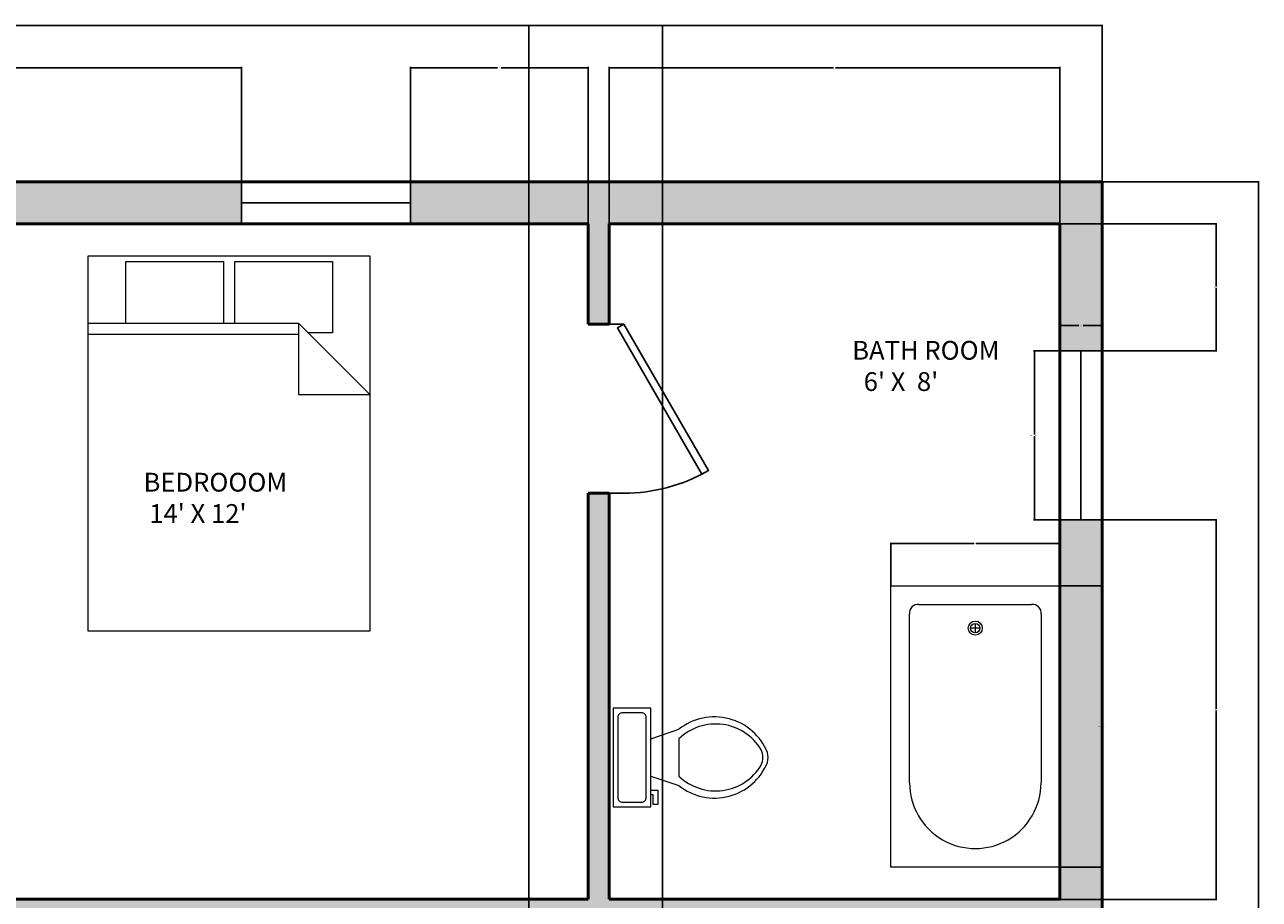
# Model space of a CAD drawing. Units: inches. Extents: x 4 to 671, y -79 to 570.
# Tile 7 of 7: x 408 to 671, y 383 to 570. Entities that reach past the tile are written whole.
import ezdxf

# ---------------------------------------------------------------- set-up
doc = ezdxf.new("R2010")
doc.units = ezdxf.units.IN
doc.header["$MEASUREMENT"] = 0
for name, color, linetype, lineweight in [('A-ANNO-DIMS', 2, 'Continuous', 18), ('A-AREA-IDEN', 7, 'Continuous', 18), ('A-WALL', 7, 'Continuous', 50), ('A-WALL-PATT', 251, 'Continuous', 13), ('bathroom', 90, 'Continuous', 18), ('doors', 40, 'Continuous', 25), ('furniture', 220, 'Continuous', 18), ('window', 30, 'Continuous', 25)]:
    doc.layers.add(name, color=color, linetype=linetype, lineweight=lineweight)
doc.styles.get("Standard").update_dxf_attribs({"font": 'arial.ttf'})
doc.dimstyles.get("Standard").update_dxf_attribs({"dimtxt": 0.18, "dimasz": 0.18, "dimexe": 0.18, "dimexo": 0.0625, "dimgap": 0.09, "dimtad": 0, "dimtih": 1, "dimtoh": 1, "dimdec": 4, "dimzin": 0, "dimdsep": 46, "dimtxsty": 'Standard', "dimcen": 0.09, "dimadec": 0, "dimazin": 0, "dimtfac": 1, "dimtdec": 4, "dimtofl": 0, "dimtmove": 0, "dimatfit": 3, "dimfxl": 1, "dimtolj": 1, "dimtzin": 0, "dimarcsym": 0})

# ---------------------------------------------------------------- blocks, each defined once
blk = doc.blocks.new('*U9')
for p, q in [((0, 0), (0, -6)), ((40, 0), (40, -6))]:
    blk.add_line(p, q)
blk.add_lwpolyline([(0, 0), (34.64, 20), (35.52, 18.48), (0.87, -1.52)], close=True)
blk.add_arc((0, 0), 40, 0, 30)
blk = doc.blocks.new('Bath Tub - 26 x 60 in.')
for p, q in [((8, -18), (10, -18)), ((9, -17), (9, -19))]:
    blk.add_line(p, q)
blk.add_lwpolyline([(0, -36), (0, 0), (60, 0), (60, -36)], close=True)
for points in [[(6, -4), (42, -4)], [(4, -30), (4, -6)], [(42, -32), (6, -32)]]:
    blk.add_lwpolyline(points)
for radius in [1.5, 1]:
    blk.add_circle((9, -18), radius)
for centre, radius, start, end in [((5.75, -5.75), 1.77, 81.8699, 188.1301), ((42, -18), 14, 270, 90), ((5.75, -30.25), 1.77, 171.8699, 278.1301)]:
    blk.add_arc(centre, radius, start, end)
blk = doc.blocks.new('Bed - Queen')
for p, q in [((0, -80.00003), (0, 0)), ((0, 0), (59.99999, 0)), ((59.99999, 0), (59.99999, -80.00003)), ((7.99999, -1.2), (28.79998, -1.2)), ((7.99999, -14.4), (7.99999, -1.2)), ((28.79998, -1.2), (28.79998, -14.4)), ((31.19999, -1.2), (51.99999, -1.2)), ((31.19999, -14.4), (31.19999, -1.2)), ((51.99999, -1.2), (51.99999, -16.4)), ((0, -14.4), (44.8, -14.4)), ((59.99999, -29.6), (44.8, -14.4)), ((44.8, -14.4), (44.8, -29.6)), ((44.8, -16.8), (0, -16.8)), ((51.99999, -16.4), (46.79936, -16.4)), ((44.8, -29.6), (59.99999, -29.6)), ((59.99999, -80.00003), (0, -80.00003))]:
    blk.add_line(p, q)
blk = doc.blocks.new('Toilet - top')
for p, q in [((9.5, -6), (9.5, -2)), ((-10, -8.5), (-8, -8.5)), ((-10, -9.5), (-10, -8.5)), ((-7, -9.5), (-10, -9.5)), ((-8, -8.5), (-8, -8)), ((-7, -8), (-7, -9.5)), ((-4, -8), (-6, -14)), ((4, -8), (6, -14)), ((4, -14), (-4, -14))]:
    blk.add_line(p, q)
blk.add_lwpolyline([(10.5, -8), (10.5, 0), (-10.5, 0), (-10.5, -8)], close=True)
for points in [[(-9.5, -2), (-9.5, -6)], [(8.5, -1), (-8.5, -1)], [(-8.5, -7), (8.5, -7)]]:
    blk.add_lwpolyline(points)
for centre, radius, start, end in [((-8.62, -1.88), 0.884, 81.8699, 188.1301), ((8.62, -1.88), 0.884, 351.8699, 98.1301), ((-8.62, -6.12), 0.884, 171.8699, 278.1301), ((8.62, -6.12), 0.884, 261.8699, 8.1301), ((3.52, -21.58), 12.17, 141.4691, 247.9714), ((4.2, -21.82), 11.33, 136.3677, 238.9468), ((-3.52, -21.58), 12.17, 292.0284, 38.5307), ((-4.2, -21.82), 11.33, 301.053, 43.6321), ((0, -27.88), 4, 245.7318, 294.2682), ((0, -29), 4, 254.8605, 285.1395)]:
    blk.add_arc(centre, radius, start, end)
blk = doc.blocks.new('WIN-36')
for p, q in [((0, 0), (0, 9)), ((0, 9), (36, 9)), ((36, 9), (36, 0)), ((36, 9), (36, 4.5)), ((36, 4.5), (0, 4.5)), ((36, 0), (0, 0))]:
    blk.add_line(p, q)
blk = doc.blocks.new('WIN-36-EAST')
for p, q in [((9, 36), (0, 36)), ((0, 36), (0, 0)), ((4.5, 0), (4.5, 36)), ((9, 0), (9, 36)), ((0, 0), (9, 0)), ((0, 0), (4.5, 0))]:
    blk.add_line(p, q)
blk = doc.blocks.new('*D23')
at = {"layer": 'A-ANNO-DIMS', "color": 0, "lineweight": -2, "transparency": 16777216}
for p, q in [((628.38, 500.27), (622.86, 500.27)), ((623.04, 500.09), (623.04, 482.45)), ((623.04, 464.45), (623.04, 482.08)), ((628.38, 464.27), (622.86, 464.27))]:
    blk.add_line(p, q, dxfattribs=at)
at = {"layer": 'A-ANNO-DIMS', "color": 0, "transparency": 16777216}
for points in [[(623.01, 500.09), (623.07, 500.09), (623.04, 500.27)], [(623.01, 464.45), (623.07, 464.45), (623.04, 464.27)]]:
    blk.add_solid(points, dxfattribs=at)
at = {"layer": 'Defpoints', "color": 0, "transparency": 16777216}
for p in [(623.04, 500.27), (628.44, 500.27), (628.44, 464.27)]:
    blk.add_point(p, dxfattribs=at)
at = {"layer": 'A-ANNO-DIMS', "color": 0, "transparency": 16777216, "insert": (623.04, 482.27), "char_height": 0.18, "attachment_point": 5}
blk.add_mtext('\\A1;WINDOW 36 TYP.', dxfattribs=at)
blk = doc.blocks.new('*D24')
at = {"layer": 'A-ANNO-DIMS', "color": 0, "lineweight": -2, "transparency": 16777216}
for p, q in [((628.44, 500.33), (628.44, 505.85)), ((628.62, 505.67), (632.48, 505.67)), ((637.26, 505.67), (633.4, 505.67)), ((637.44, 500.33), (637.44, 505.85))]:
    blk.add_line(p, q, dxfattribs=at)
at = {"layer": 'A-ANNO-DIMS', "color": 0, "transparency": 16777216}
for points in [[(628.62, 505.7), (628.62, 505.64), (628.44, 505.67)], [(637.26, 505.7), (637.26, 505.64), (637.44, 505.67)]]:
    blk.add_solid(points, dxfattribs=at)
at = {"layer": 'Defpoints', "color": 0, "transparency": 16777216}
for p in [(637.44, 505.67), (628.44, 500.27), (637.44, 500.27)]:
    blk.add_point(p, dxfattribs=at)
at = {"layer": 'A-ANNO-DIMS', "color": 0, "transparency": 16777216, "insert": (632.94, 505.67), "char_height": 0.18, "attachment_point": 5}
blk.add_mtext('\\A1;9 TYP.', dxfattribs=at)
blk = doc.blocks.new('*D45')
at = {"layer": 'A-ANNO-DIMS', "color": 0, "lineweight": -2, "transparency": 16777216}
for p, q in [((628.5, 450.18), (637.62, 450.18)), ((637.44, 450), (637.44, 420.36)), ((637.44, 390.36), (637.44, 420)), ((628.5, 390.18), (637.62, 390.18))]:
    blk.add_line(p, q, dxfattribs=at)
at = {"layer": 'A-ANNO-DIMS', "color": 0, "transparency": 16777216}
for points in [[(637.41, 450), (637.47, 450), (637.44, 450.18)], [(637.41, 390.36), (637.47, 390.36), (637.44, 390.18)]]:
    blk.add_solid(points, dxfattribs=at)
at = {"layer": 'Defpoints', "color": 0, "transparency": 16777216}
for p in [(628.44, 450.18), (628.44, 390.18), (637.44, 390.18)]:
    blk.add_point(p, dxfattribs=at)
at = {"layer": 'A-ANNO-DIMS', "color": 0, "transparency": 16777216, "insert": (637.44, 420.18), "char_height": 0.18, "attachment_point": 5}
blk.add_mtext('\\A1;BATHTUB 60', dxfattribs=at)
blk = doc.blocks.new('*D46')
at = {"layer": 'A-ANNO-DIMS', "color": 0, "lineweight": -2, "transparency": 16777216}
for p, q in [((592.44, 450.24), (592.44, 459.36)), ((592.62, 459.18), (610.22, 459.18)), ((628.26, 459.18), (610.66, 459.18)), ((628.44, 450.24), (628.44, 459.36))]:
    blk.add_line(p, q, dxfattribs=at)
at = {"layer": 'A-ANNO-DIMS', "color": 0, "transparency": 16777216}
for points in [[(592.62, 459.21), (592.62, 459.15), (592.44, 459.18)], [(628.26, 459.21), (628.26, 459.15), (628.44, 459.18)]]:
    blk.add_solid(points, dxfattribs=at)
at = {"layer": 'Defpoints', "color": 0, "transparency": 16777216}
for p in [(628.44, 459.18), (592.44, 450.18), (628.44, 450.18)]:
    blk.add_point(p, dxfattribs=at)
at = {"layer": 'A-ANNO-DIMS', "color": 0, "transparency": 16777216, "insert": (610.44, 459.18), "char_height": 0.18, "attachment_point": 5}
blk.add_mtext('\\A1;36', dxfattribs=at)
blk = doc.blocks.new('*D49')
at = {"layer": 'A-ANNO-DIMS', "color": 0, "lineweight": -2, "transparency": 16777216}
for p, q in [((37.44, 536.41), (37.44, 569.83)), ((37.62, 569.65), (337.15, 569.65)), ((637.26, 569.65), (337.73, 569.65)), ((637.44, 536.41), (637.44, 569.83))]:
    blk.add_line(p, q, dxfattribs=at)
at = {"layer": 'A-ANNO-DIMS', "color": 0, "transparency": 16777216}
for points in [[(37.62, 569.68), (37.62, 569.62), (37.44, 569.65)], [(637.26, 569.68), (637.26, 569.62), (637.44, 569.65)]]:
    blk.add_solid(points, dxfattribs=at)
at = {"layer": 'Defpoints', "color": 0, "transparency": 16777216}
for p in [(637.44, 569.65), (37.44, 536.35), (637.44, 536.35)]:
    blk.add_point(p, dxfattribs=at)
at = {"layer": 'A-ANNO-DIMS', "color": 0, "transparency": 16777216, "insert": (337.44, 569.65), "char_height": 0.18, "attachment_point": 5}
blk.add_mtext('\\A1;600', dxfattribs=at)
blk = doc.blocks.new('*D50')
at = {"layer": 'A-ANNO-DIMS', "color": 0, "lineweight": -2, "transparency": 16777216}
for p, q in [((637.5, 536.35), (670.92, 536.35)), ((670.74, 536.17), (670.74, 245.53)), ((670.74, -45.47), (670.74, 245.17)), ((389.27, -45.65), (670.92, -45.65))]:
    blk.add_line(p, q, dxfattribs=at)
at = {"layer": 'A-ANNO-DIMS', "color": 0, "transparency": 16777216}
for points in [[(670.71, 536.17), (670.77, 536.17), (670.74, 536.35)], [(670.71, -45.47), (670.77, -45.47), (670.74, -45.65)]]:
    blk.add_solid(points, dxfattribs=at)
at = {"layer": 'Defpoints', "color": 0, "transparency": 16777216}
for p in [(637.44, 536.35), (389.21, -45.65), (670.74, -45.65)]:
    blk.add_point(p, dxfattribs=at)
at = {"layer": 'A-ANNO-DIMS', "color": 0, "transparency": 16777216, "insert": (670.74, 245.35), "char_height": 0.18, "attachment_point": 5}
blk.add_mtext('\\A1;582', dxfattribs=at)
blk = doc.blocks.new('*D73')
at = {"layer": 'A-ANNO-DIMS', "color": 0, "lineweight": -2, "transparency": 16777216}
for p, q in [((628.5, 527.35), (661.92, 527.35)), ((661.74, 527.17), (661.74, 513.99)), ((661.74, 500.45), (661.74, 513.63)), ((628.5, 500.27), (661.92, 500.27))]:
    blk.add_line(p, q, dxfattribs=at)
at = {"layer": 'A-ANNO-DIMS', "color": 0, "transparency": 16777216}
for points in [[(661.71, 527.17), (661.77, 527.17), (661.74, 527.35)], [(661.71, 500.45), (661.77, 500.45), (661.74, 500.27)]]:
    blk.add_solid(points, dxfattribs=at)
at = {"layer": 'Defpoints', "color": 0, "transparency": 16777216}
for p in [(628.44, 527.35), (628.44, 500.27), (661.74, 500.27)]:
    blk.add_point(p, dxfattribs=at)
at = {"layer": 'A-ANNO-DIMS', "color": 0, "transparency": 16777216, "insert": (661.74, 513.81), "char_height": 0.18, "attachment_point": 5}
blk.add_mtext('\\A1;27.085', dxfattribs=at)
blk = doc.blocks.new('*D74')
at = {"layer": 'A-ANNO-DIMS', "color": 0, "lineweight": -2, "transparency": 16777216}
for p, q in [((628.5, 464.27), (661.92, 464.27)), ((661.74, 464.09), (661.74, 423.99)), ((661.74, 383.53), (661.74, 423.63)), ((628.5, 383.35), (661.92, 383.35))]:
    blk.add_line(p, q, dxfattribs=at)
at = {"layer": 'A-ANNO-DIMS', "color": 0, "transparency": 16777216}
for points in [[(661.71, 464.09), (661.77, 464.09), (661.74, 464.27)], [(661.71, 383.53), (661.77, 383.53), (661.74, 383.35)]]:
    blk.add_solid(points, dxfattribs=at)
at = {"layer": 'Defpoints', "color": 0, "transparency": 16777216}
for p in [(628.44, 464.27), (628.44, 383.35), (661.74, 383.35)]:
    blk.add_point(p, dxfattribs=at)
at = {"layer": 'A-ANNO-DIMS', "color": 0, "transparency": 16777216, "insert": (661.74, 423.81), "char_height": 0.18, "attachment_point": 5}
blk.add_mtext('\\A1;80.91', dxfattribs=at)
blk = doc.blocks.new('*D79')
at = {"layer": 'A-ANNO-DIMS', "color": 0, "lineweight": -2, "transparency": 16777216}
for p, q in [((532.44, 527.41), (532.44, 560.83)), ((532.62, 560.65), (580.22, 560.65)), ((628.26, 560.65), (580.66, 560.65)), ((628.44, 527.41), (628.44, 560.83))]:
    blk.add_line(p, q, dxfattribs=at)
at = {"layer": 'A-ANNO-DIMS', "color": 0, "transparency": 16777216}
for points in [[(532.62, 560.68), (532.62, 560.62), (532.44, 560.65)], [(628.26, 560.68), (628.26, 560.62), (628.44, 560.65)]]:
    blk.add_solid(points, dxfattribs=at)
at = {"layer": 'Defpoints', "color": 0, "transparency": 16777216}
for p in [(628.44, 560.65), (532.44, 527.35), (628.44, 527.35)]:
    blk.add_point(p, dxfattribs=at)
at = {"layer": 'A-ANNO-DIMS', "color": 0, "transparency": 16777216, "insert": (580.44, 560.65), "char_height": 0.18, "attachment_point": 5}
blk.add_mtext('\\A1;96', dxfattribs=at)
blk = doc.blocks.new('*D83')
at = {"layer": 'A-ANNO-DIMS', "color": 0, "lineweight": -2, "transparency": 16777216}
for p, q in [((341.11, 527.41), (341.11, 560.83)), ((341.29, 560.65), (397.17, 560.65)), ((453.95, 560.65), (398.07, 560.65)), ((454.13, 527.41), (454.13, 560.83))]:
    blk.add_line(p, q, dxfattribs=at)
at = {"layer": 'A-ANNO-DIMS', "color": 0, "transparency": 16777216}
for points in [[(341.29, 560.68), (341.29, 560.62), (341.11, 560.65)], [(453.95, 560.68), (453.95, 560.62), (454.13, 560.65)]]:
    blk.add_solid(points, dxfattribs=at)
at = {"layer": 'Defpoints', "color": 0, "transparency": 16777216}
for p in [(454.13, 560.65), (341.11, 527.35), (454.13, 527.35)]:
    blk.add_point(p, dxfattribs=at)
at = {"layer": 'A-ANNO-DIMS', "color": 0, "transparency": 16777216, "insert": (397.62, 560.65), "char_height": 0.18, "attachment_point": 5}
blk.add_mtext('\\A1;113.02', dxfattribs=at)
blk = doc.blocks.new('*D84')
at = {"layer": 'A-ANNO-DIMS', "color": 0, "lineweight": -2, "transparency": 16777216}
for p, q in [((490.13, 527.41), (490.13, 560.83)), ((490.31, 560.65), (508.66, 560.65)), ((527.76, 560.65), (509.41, 560.65)), ((527.94, 527.41), (527.94, 560.83))]:
    blk.add_line(p, q, dxfattribs=at)
at = {"layer": 'A-ANNO-DIMS', "color": 0, "transparency": 16777216}
for points in [[(490.31, 560.68), (490.31, 560.62), (490.13, 560.65)], [(527.76, 560.68), (527.76, 560.62), (527.94, 560.65)]]:
    blk.add_solid(points, dxfattribs=at)
at = {"layer": 'Defpoints', "color": 0, "transparency": 16777216}
for p in [(527.94, 560.65), (490.13, 527.35), (527.94, 527.35)]:
    blk.add_point(p, dxfattribs=at)
at = {"layer": 'A-ANNO-DIMS', "color": 0, "transparency": 16777216, "insert": (509.03, 560.65), "char_height": 0.18, "attachment_point": 5}
blk.add_mtext('\\A1;37.81', dxfattribs=at)
blk = doc.blocks.new('*D93')
at = {"layer": 'A-ANNO-DIMS', "color": 0, "lineweight": -2, "transparency": 16777216}
for p, q in [((515.3, 371.26), (515.3, 569.83)), ((515.48, 569.65), (529.17, 569.65)), ((543.64, 569.65), (529.96, 569.65)), ((543.82, 371.26), (543.82, 569.83))]:
    blk.add_line(p, q, dxfattribs=at)
at = {"layer": 'A-ANNO-DIMS', "color": 0, "transparency": 16777216}
for points in [[(515.48, 569.68), (515.48, 569.62), (515.3, 569.65)], [(543.64, 569.68), (543.64, 569.62), (543.82, 569.65)]]:
    blk.add_solid(points, dxfattribs=at)
at = {"layer": 'Defpoints', "color": 0, "transparency": 16777216}
for p in [(543.82, 569.65), (515.3, 371.2), (543.82, 371.2)]:
    blk.add_point(p, dxfattribs=at)
at = {"layer": 'A-ANNO-DIMS', "color": 0, "transparency": 16777216, "insert": (529.56, 569.65), "char_height": 0.18, "attachment_point": 5}
blk.add_mtext('\\A1;28.53', dxfattribs=at)

msp = doc.modelspace()

# ---------------------------------------------------------------- hatches: boundary and pattern name
at = {"layer": 'A-WALL-PATT'}
h = msp.add_hatch(color=256, dxfattribs=at)
h.dxf.hatch_style = 1
h.paths.add_polyline_path([(206.5642, 536.3513), (93.0095, 536.3513), (93.0095, 531.8513), (93.0095, 527.3513), (118.4392, 527.3513), (118.4392, 443.3513), (115.4392, 443.3513), (115.4392, 438.8513), (118.4392, 438.8513), (118.4392, 422.3513), (120.6892, 422.3513), (122.9392, 422.3513), (122.9392, 527.3513), (206.5642, 527.3513)])
h.paths.add_polyline_path([(305.1113, 536.3513), (242.5642, 536.3513), (242.5642, 531.8513), (242.5642, 527.3513), (290.9392, 527.3513), (290.9392, 422.3513), (293.1892, 422.3513), (295.4392, 422.3513), (295.4392, 438.8513), (301.4392, 438.8513), (301.4392, 443.3513), (295.4392, 443.3513), (295.4392, 527.3513), (305.1113, 527.3513)])
h.paths.add_polyline_path([(454.1293, 536.3513), (341.1113, 536.3513), (341.1113, 531.8513), (341.1113, 527.3513), (355.4392, 527.3513), (355.4392, 443.3513), (325.4392, 443.3513), (325.4392, 438.8513), (355.4392, 438.8513), (355.4392, 422.3513), (359.9392, 422.3513), (359.9392, 527.3513), (454.1293, 527.3513)])
h.paths.add_polyline_path([(637.4392, 536.3513), (490.1293, 536.3513), (490.1293, 531.8513), (490.1293, 527.3513), (527.9392, 527.3513), (527.9392, 505.9443), (532.4392, 505.9443), (532.4392, 527.3513), (628.4392, 527.3513), (628.4392, 500.2662), (637.4392, 500.2662)])
h.paths.add_polyline_path([(637.4392, 464.2662), (628.4392, 464.2662), (628.4392, 383.3513), (556.4392, 383.3513), (532.4392, 383.3513), (532.4392, 469.9443), (527.9392, 469.9443), (527.9392, 383.3513), (359.9392, 383.3513), (359.9392, 386.3513), (355.4392, 386.3513), (355.4392, 378.8513), (403.4392, 378.8513), (403.4392, 318.8513), (407.9392, 318.8513), (407.9392, 378.8513), (551.9392, 378.8513), (551.9392, 290.3513), (554.1892, 290.3513, -0.01563646), (556.4392, 290.2809), (556.4392, 378.8513), (628.4392, 378.8513), (628.4392, 342.8513), (637.4392, 342.8513)])

# ---------------------------------------------------------------- linework, layer by layer
at = {"layer": 'A-WALL'}
for p, q in [((359.9392, 527.3513), (527.9392, 527.3513)), ((527.9392, 505.9443), (527.9392, 527.3513)), ((532.4392, 527.3513), (628.4392, 527.3513)), ((532.4392, 505.9443), (532.4392, 527.3513)), ((628.4392, 527.3513), (628.4392, 383.3513)), ((527.9392, 505.9443), (532.4392, 505.9443)), ((527.9392, 383.3513), (527.9392, 469.9443)), ((527.9392, 469.9443), (532.4392, 469.9443)), ((532.4392, 383.3513), (532.4392, 469.9443)), ((359.9392, 383.3513), (527.9392, 383.3513)), ((532.4392, 383.3513), (628.4392, 383.3513)), ((556.4392, 383.3513), (628.4392, 383.3513))]:
    msp.add_line(p, q, dxfattribs=at)
msp.add_lwpolyline([(313.4392, 56.3513), (37.4392, 56.3513), (37.4392, 536.3513), (637.4392, 536.3513), (637.4392, 56.3513), (362.9392, 56.3513)], dxfattribs=at)

# ---------------------------------------------------------------- block references
at = {"layer": 'bathroom'}
for name, p, rotation in [('Bath Tub - 26 x 60 in.', (628.4392, 450.1793), 270), ('Toilet - top', (533.3163, 413.595), 90)]:
    msp.add_blockref(name, p, dxfattribs=dict(at, rotation=rotation))
at = {"layer": 'doors', "xscale": 0.9, "yscale": 0.9, "zscale": 0.9, "rotation": 270}
msp.add_blockref('*U9', (535.5892, 505.9443), dxfattribs=at)
at = {"layer": 'furniture'}
msp.add_blockref('Bed - Queen', (421.4809, 520.558), dxfattribs=at)
at = {"layer": 'window'}
for name, p in [('WIN-36', (454.129, 527.351)), ('WIN-36-EAST', (628.439, 464.2658))]:
    msp.add_blockref(name, p, dxfattribs=at)

# ---------------------------------------------------------------- texts
at = {"layer": 'A-AREA-IDEN', "char_height": 4, "attachment_point": 1}
for s, insert in [("BATH ROOM\\P  6' X  8'", (584.2255, 502.4052)), ("BEDROOOM\\P 14' X 12'", (433.2638, 474.2826))]:
    msp.add_mtext_dynamic_manual_height_columns(s, width=44.806469, gutter_width=1, heights=[0], dxfattribs=dict(at, insert=insert))

# ---------------------------------------------------------------- dimensions: what is measured, and where the dimension line sits
at = {"layer": 'A-ANNO-DIMS'}
for base, p1, p2, override, picture, middle in [((637.4392, 569.6513), (37.4392, 536.3513), (637.4392, 536.3513), {"dimdec": 0, "dimlfac": 1, "dimrnd": 0, "dimzin": 0, "dimdsep": 46, "dimlunit": 2}, '*D49', (337.4392, 569.6513)), ((543.8249, 569.6513), (515.2973, 371.2019), (543.8249, 371.2019), {"dimdec": 2, "dimlfac": 1, "dimrnd": 0, "dimzin": 0, "dimdsep": 46, "dimlunit": 2}, '*D93', (529.5611, 569.6513)), ((454.1293, 560.6513), (341.1113, 527.3513), (454.1293, 527.3513), {"dimdec": 2, "dimlfac": 1, "dimrnd": 0, "dimzin": 0, "dimdsep": 46, "dimlunit": 2}, '*D83', (397.6203, 560.6513)), ((527.9392, 560.6513), (490.1293, 527.3513), (527.9392, 527.3513), {"dimdec": 2, "dimlfac": 1, "dimrnd": 0, "dimzin": 0, "dimdsep": 46, "dimlunit": 2}, '*D84', (509.0343, 560.6513)), ((628.4392, 560.6513), (532.4392, 527.3513), (628.4392, 527.3513), {"dimdec": 0, "dimlfac": 1, "dimrnd": 0, "dimzin": 0, "dimdsep": 46, "dimlunit": 2}, '*D79', (580.4392, 560.6513)), ((628.4392, 459.1793), (592.4392, 450.1793), (628.4392, 450.1793), {"dimdec": 0, "dimlfac": 1, "dimrnd": 0, "dimzin": 0, "dimdsep": 46, "dimlunit": 2}, '*D46', (610.4392, 459.1793))]:
    dim = msp.add_linear_dim(base=base, p1=p1, p2=p2, dimstyle='Standard', override=override, dxfattribs=at)
    dim.commit()
    dim.dimension.update_dxf_attribs({"geometry": picture, "text_midpoint": middle})
for base, p1, p2, angle, override, picture, middle in [((670.7392, -45.6487), (637.4392, 536.3513), (389.2077, -45.6487), 90, {"dimdec": 0, "dimlfac": 1, "dimrnd": 0, "dimzin": 0, "dimdsep": 46, "dimlunit": 2}, '*D50', (670.7392, 245.3513)), ((661.7392, 500.2662), (628.4392, 527.3513), (628.4392, 500.2662), 270, {"dimdec": 3, "dimlfac": 1, "dimrnd": 0, "dimzin": 0, "dimdsep": 46, "dimlunit": 2}, '*D73', (661.7392, 513.8087)), ((661.7392, 383.3513), (628.4392, 464.2662), (628.4392, 383.3513), 270, {"dimdec": 2, "dimlfac": 1, "dimrnd": 0, "dimzin": 0, "dimdsep": 46, "dimlunit": 2}, '*D74', (661.7392, 423.8087))]:
    dim = msp.add_linear_dim(base=base, p1=p1, p2=p2, angle=angle, dimstyle='Standard', override=override, dxfattribs=at)
    dim.commit()
    dim.dimension.update_dxf_attribs({"geometry": picture, "text_midpoint": middle})
dim = msp.add_linear_dim(base=(637.4392, 505.6662), p1=(628.4392, 500.2662), p2=(637.4392, 500.2662), text='<> TYP.', dimstyle='Standard', override={"dimdec": 0, "dimlfac": 1, "dimrnd": 0, "dimzin": 0, "dimdsep": 46, "dimlunit": 2}, dxfattribs=at)
dim.commit()
dim.dimension.update_dxf_attribs({"geometry": '*D24', "text_midpoint": (632.9392, 505.6662)})
for base, p1, p2, angle, text, picture, middle in [((623.0392, 500.2662), (628.4392, 464.2662), (628.4392, 500.2662), 90, 'WINDOW <> TYP.', '*D23', (623.0392, 482.2662)), ((637.4392, 390.1793), (628.4392, 450.1793), (628.4392, 390.1793), 270, 'BATHTUB <>', '*D45', (637.4392, 420.1793))]:
    dim = msp.add_linear_dim(base=base, p1=p1, p2=p2, angle=angle, text=text, dimstyle='Standard', override={"dimdec": 0, "dimlfac": 1, "dimrnd": 0, "dimzin": 0, "dimdsep": 46, "dimlunit": 2}, dxfattribs=at)
    dim.commit()
    dim.dimension.update_dxf_attribs({"geometry": picture, "text_midpoint": middle})

doc.saveas('drawing.dxf')
